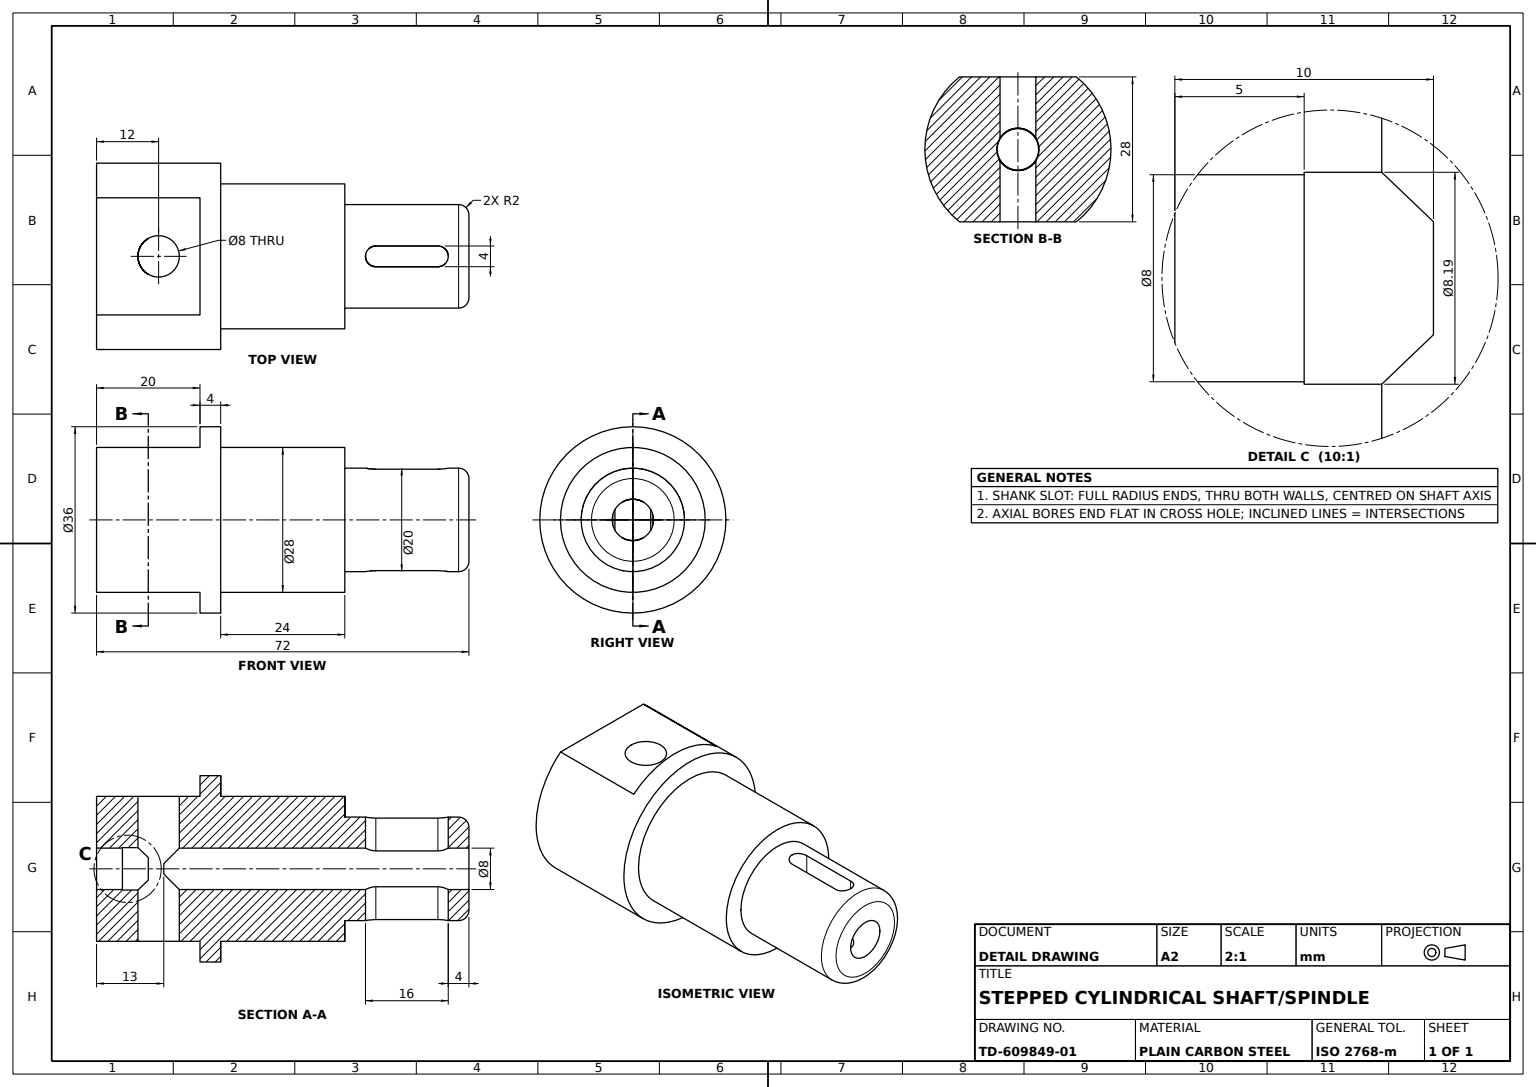
from build123d import *

# Parameters (mm, degrees)
SHANK_20_SKETCH_R          = 10
SHANK_20_STEP_1_DEPTH      = 8
SHANK_STEP_2_SKETCH_R      = 10
SHANK_20_STEP_2_DEPTH      = 8
SHANK_STEP_3_SKETCH_R      = 10
SHANK_20_STEP_3_DEPTH      = 8
SHANK_END_FILLET_R2_R      = 2
SHANK_BORE_8_SKETCH_R      = 4
SHANK_BORE_8_CUT_1_DEPTH   = 8
SHANK_BORE_CUT_2_SKETCH_R  = 4
SHANK_BORE_8_CUT_2_DEPTH   = 8
SHANK_BORE_CUT_3_SKETCH_R  = 4
SHANK_BORE_8_CUT_3_DEPTH   = 18
COLLAR_28_SKETCH_R         = 14
COLLAR_28_STEP_1_DEPTH     = 8
COLLAR_STEP_2_SKETCH_R     = 14
COLLAR_28_STEP_2_DEPTH     = 8
COLLAR_STEP_3_SKETCH_R     = 14
COLLAR_28_STEP_3_DEPTH     = 8
HEAD_36_SKETCH_R           = 18
HEAD_36_STEP_1_DEPTH       = 8
HEAD_STEP_2_SKETCH_R       = 18
HEAD_36_STEP_2_DEPTH       = 8
HEAD_STEP_3_SKETCH_R       = 18
HEAD_36_STEP_3_DEPTH       = 8
HEAD_FLAT_DEPTH            = 51
HEAD_FLAT_DEPTH_BACK       = 40
HEAD_FLAT_SKETCH_W         = 4
HEAD_FLAT_SKETCH_H         = 20
CROSS_HOLE_8_DEPTH         = 20
CROSS_HOLE_8_DEPTH_BACK    = 52
CROSS_HOLE_8_SKETCH_R      = 4
COLLAR_BORE_CUT_1_SKETCH_R = 4
COLLAR_BORE_CUT_1_DEPTH    = 5
COLLAR_BORE_CUT_2_SKETCH_R = 4
COLLAR_BORE_CUT_2_DEPTH    = 5
COLLAR_BORE_CUT_3_SKETCH_R = 4
COLLAR_BORE_CUT_3_DEPTH    = 5
HEAD_START                 = -5
HEAD_BORE_8_SKETCH_R       = 4
HEAD_BORE_8_CUT_1_DEPTH    = 5
HEAD_BORE_CUT_2_SKETCH_R   = 4.094669118
HEAD_BORE_8_CUT_2_DEPTH    = 5
COLLAR_BORE_CUT_4_SKETCH_R = 4
COLLAR_BORE_CUT_4_DEPTH    = 5
INNER_BORE_8_SKETCH_R      = 4
INNER_BORE_8_CUT_1_DEPTH   = 5
INNER_BORE_CUT_2_SKETCH_R  = 4
INNER_BORE_8_CUT_2_DEPTH   = 5
INNER_BORE_CUT_3_SKETCH_R  = 4
INNER_BORE_8_CUT_3_DEPTH   = 5
SHANK_SLOT_DEPTH           = 137
SHANK_SLOT_DEPTH_BACK      = 146


with BuildPart() as part:
    # Shank Ø20 Sketch → Shank Ø20 Step 1 (new body)
    with BuildSketch(Plane(origin=(0, 0, 0), x_dir=(1, 0, 0), z_dir=(0, 1, 0))):
        with Locations(Location((0, 0, 0), (0, 0, 270))):
            Circle(SHANK_20_SKETCH_R)
    extrude(amount=SHANK_20_STEP_1_DEPTH)

    # Shank Step 2 Sketch → Shank Ø20 Step 2 (add)
    with BuildSketch(Plane(origin=(0, 8, 0), x_dir=(1, 0, 0), z_dir=(0, 1, 0))):
        with Locations(Location((0, 0, 0), (0, 0, 270))):
            Circle(SHANK_STEP_2_SKETCH_R)
    extrude(amount=SHANK_20_STEP_2_DEPTH)

    # Shank Step 3 Sketch → Shank Ø20 Step 3 (add)
    with BuildSketch(Plane(origin=(0, 16, 0), x_dir=(1, 0, 0), z_dir=(0, 1, 0))):
        with Locations(Location((0, 0, 0), (0, 0, 270))):
            Circle(SHANK_STEP_3_SKETCH_R)
    extrude(amount=SHANK_20_STEP_3_DEPTH)

    # Shank End Fillet R2
    shank_end_fillet_r2_edges = [part.edges().sort_by_distance(p)[0] for p in [
        (0, 24, -10),
    ]]
    fillet(shank_end_fillet_r2_edges, radius=SHANK_END_FILLET_R2_R)

    # Shank Bore Ø8 Sketch → Shank Bore Ø8 Cut 1 (cut)
    with BuildSketch(Plane(origin=(0, 24, 0), x_dir=(1, 0, 0), z_dir=(0, 1, 0))):
        with Locations(Location((0, 0, 0), (0, 0, 270))):
            Circle(SHANK_BORE_8_SKETCH_R)
    extrude(amount=-SHANK_BORE_8_CUT_1_DEPTH, mode=Mode.SUBTRACT)

    # Shank Bore Cut 2 Sketch → Shank Bore Ø8 Cut 2 (cut)
    with BuildSketch(Plane(origin=(0, 16, 0), x_dir=(1, 0, 0), z_dir=(0, 1, 0))):
        with Locations(Location((0, 0, 0), (0, 0, 270))):
            Circle(SHANK_BORE_CUT_2_SKETCH_R)
    extrude(amount=-SHANK_BORE_8_CUT_2_DEPTH, mode=Mode.SUBTRACT)

    # Shank Bore Cut 3 Sketch → Shank Bore Ø8 Cut 3 (cut)
    with BuildSketch(Plane(origin=(0, 8, 0), x_dir=(1, 0, 0), z_dir=(0, 1, 0))):
        with Locations(Location((0, 0, 0), (0, 0, 270))):
            Circle(SHANK_BORE_CUT_3_SKETCH_R)
    extrude(amount=-SHANK_BORE_8_CUT_3_DEPTH, mode=Mode.SUBTRACT)

    # Collar Ø28 Sketch → Collar Ø28 Step 1 (add)
    with BuildSketch(Plane.XZ):
        with Locations(Location((0, 0, 0), (0, 0, 270))):
            Circle(COLLAR_28_SKETCH_R)
    extrude(amount=COLLAR_28_STEP_1_DEPTH)

    # Collar Step 2 Sketch → Collar Ø28 Step 2 (add)
    with BuildSketch(Plane.XZ.offset(8)):
        with Locations(Location((0, 0, 0), (0, 0, 270))):
            Circle(COLLAR_STEP_2_SKETCH_R)
    extrude(amount=COLLAR_28_STEP_2_DEPTH)

    # Collar Step 3 Sketch → Collar Ø28 Step 3 (add)
    with BuildSketch(Plane.XZ.offset(16)):
        with Locations(Location((0, 0, 0), (0, 0, 270))):
            Circle(COLLAR_STEP_3_SKETCH_R)
    extrude(amount=COLLAR_28_STEP_3_DEPTH)

    # Head Ø36 Sketch → Head Ø36 Step 1 (add)
    with BuildSketch(Plane.XZ.offset(24)):
        with Locations(Location((0, 0, 0), (0, 0, 270))):
            Circle(HEAD_36_SKETCH_R)
    extrude(amount=HEAD_36_STEP_1_DEPTH)

    # Head Step 2 Sketch → Head Ø36 Step 2 (add)
    with BuildSketch(Plane.XZ.offset(32)):
        with Locations(Location((0, 0, 0), (0, 0, 270))):
            Circle(HEAD_STEP_2_SKETCH_R)
    extrude(amount=HEAD_36_STEP_2_DEPTH)

    # Head Step 3 Sketch → Head Ø36 Step 3 (add)
    with BuildSketch(Plane.XZ.offset(40)):
        with Locations(Location((0, 0, 0), (0, 0, 270))):
            Circle(HEAD_STEP_3_SKETCH_R)
    extrude(amount=HEAD_36_STEP_3_DEPTH)

    # Head Flat Sketch → Head Flat (cut, two sides: drawn at the far end of the back side and taken through both)
    with BuildSketch(Plane.XY.offset(-HEAD_FLAT_DEPTH_BACK)):
        with Locations((-16, -38)):
            Rectangle(HEAD_FLAT_SKETCH_W, HEAD_FLAT_SKETCH_H)
        with Locations((16, -38)):
            Rectangle(HEAD_FLAT_SKETCH_W, HEAD_FLAT_SKETCH_H)
    extrude(amount=HEAD_FLAT_DEPTH + HEAD_FLAT_DEPTH_BACK, mode=Mode.SUBTRACT)

    # Cross Hole Ø8 Sketch → Cross Hole Ø8 (cut, two sides: drawn at the far end of the back side and taken through both)
    with BuildSketch(Plane(origin=(14, 0, 0), x_dir=(0, 0, -1), z_dir=(1, 0, 0)).offset(-CROSS_HOLE_8_DEPTH_BACK)):
        with Locations(Location((0, -36, 0), (0, 0, 270))):
            Circle(CROSS_HOLE_8_SKETCH_R)
    extrude(amount=CROSS_HOLE_8_DEPTH + CROSS_HOLE_8_DEPTH_BACK, mode=Mode.SUBTRACT)

    # Collar Bore Cut 1 Sketch → Collar Bore Cut 1 (cut)
    with BuildSketch(Plane(origin=(0, 0, 0), x_dir=(1, 0, 0), z_dir=(0, 1, 0))):
        with Locations(Location((0, 0, 0), (0, 0, 270))):
            Circle(COLLAR_BORE_CUT_1_SKETCH_R)
    extrude(amount=-COLLAR_BORE_CUT_1_DEPTH, mode=Mode.SUBTRACT)

    # Collar Bore Cut 2 Sketch → Collar Bore Cut 2 (cut)
    with BuildSketch(Plane(origin=(0, -5, 0), x_dir=(1, 0, 0), z_dir=(0, 1, 0))):
        with Locations(Location((0, 0, 0), (0, 0, 270))):
            Circle(COLLAR_BORE_CUT_2_SKETCH_R)
    extrude(amount=-COLLAR_BORE_CUT_2_DEPTH, mode=Mode.SUBTRACT)

    # Collar Bore Cut 3 Sketch → Collar Bore Cut 3 (cut)
    with BuildSketch(Plane(origin=(0, -10, 0), x_dir=(1, 0, 0), z_dir=(0, 1, 0))):
        with Locations(Location((0, 0, 0), (0, 0, 270))):
            Circle(COLLAR_BORE_CUT_3_SKETCH_R)
    extrude(amount=-COLLAR_BORE_CUT_3_DEPTH, mode=Mode.SUBTRACT)

    # Head Bore Ø8 Sketch → Head Bore Ø8 Cut 1 (cut)
    with BuildSketch(Plane.XZ.offset(48).offset(HEAD_START)):
        with Locations(Location((0, 0, 0), (0, 0, 90))):
            Circle(HEAD_BORE_8_SKETCH_R)
    extrude(amount=HEAD_BORE_8_CUT_1_DEPTH, mode=Mode.SUBTRACT)

    # Head Bore Cut 2 Sketch → Head Bore Ø8 Cut 2 (cut)
    with BuildSketch(Plane.XZ.offset(43)):
        with Locations(Location((0, 0, 0), (0, 0, 270))):
            Circle(HEAD_BORE_CUT_2_SKETCH_R)
    extrude(amount=-HEAD_BORE_8_CUT_2_DEPTH, mode=Mode.SUBTRACT)

    # Collar Bore Cut 4 Sketch → Collar Bore Cut 4 (cut)
    with BuildSketch(Plane(origin=(0, -15, 0), x_dir=(1, 0, 0), z_dir=(0, 1, 0))):
        with Locations(Location((0, 0, 0), (0, 0, 270))):
            Circle(COLLAR_BORE_CUT_4_SKETCH_R)
    extrude(amount=-COLLAR_BORE_CUT_4_DEPTH, mode=Mode.SUBTRACT)

    # Inner Bore Ø8 Sketch → Inner Bore Ø8 Cut 1 (cut)
    with BuildSketch(Plane(origin=(0, -20, 0), x_dir=(1, 0, 0), z_dir=(0, 1, 0))):
        with Locations(Location((0, 0, 0), (0, 0, 270))):
            Circle(INNER_BORE_8_SKETCH_R)
    extrude(amount=-INNER_BORE_8_CUT_1_DEPTH, mode=Mode.SUBTRACT)

    # Inner Bore Cut 2 Sketch → Inner Bore Ø8 Cut 2 (cut)
    with BuildSketch(Plane(origin=(0, -25, 0), x_dir=(1, 0, 0), z_dir=(0, 1, 0))):
        with Locations(Location((0, 0, 0), (0, 0, 270))):
            Circle(INNER_BORE_CUT_2_SKETCH_R)
    extrude(amount=-INNER_BORE_8_CUT_2_DEPTH, mode=Mode.SUBTRACT)

    # Inner Bore Cut 3 Sketch → Inner Bore Ø8 Cut 3 (cut)
    with BuildSketch(Plane(origin=(0, -30, 0), x_dir=(1, 0, 0), z_dir=(0, 1, 0))):
        with Locations(Location((0, 0, 0), (0, 0, 270))):
            Circle(INNER_BORE_CUT_3_SKETCH_R)
    extrude(amount=-INNER_BORE_8_CUT_3_DEPTH, mode=Mode.SUBTRACT)

    # Shank Slot Sketch → Shank Slot (cut, two sides: drawn at the far end of the back side and taken through both)
    with BuildSketch(Plane(origin=(14, 0, 0), x_dir=(0, 0, -1), z_dir=(1, 0, 0)).offset(-SHANK_SLOT_DEPTH_BACK)):
        with BuildLine():
            Line((-2, 18), (-2, 6))
            ThreePointArc((-2, 6), (0, 4), (2, 6))
            Line((2, 6), (2, 18))
            ThreePointArc((2, 18), (0, 20), (-2, 18))
        make_face()
    extrude(amount=SHANK_SLOT_DEPTH + SHANK_SLOT_DEPTH_BACK, mode=Mode.SUBTRACT)


solid = part.part
